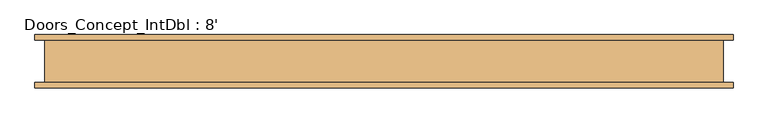
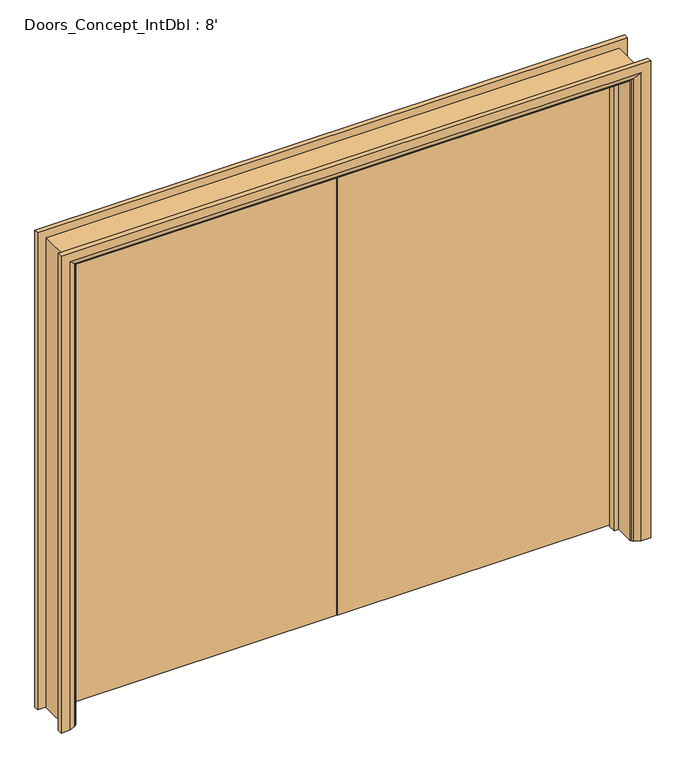
"""IFC4 building model written with IfcOpenShell, lengths in millimetres: door geometry, Doors_Concept_IntDbl : 8'."""

from ifc_helpers import new_model, si_unit, frame, origin, place, context, project, spatial, polyline, circle_curve, ellipse_curve, outline, extrude, faceted_brep, source, transform, mapped, element, save
from ifc_brep_helpers import plane_surface, cylinder_surface, advanced_brep


def doors_concept_intdbl_8_5090a96f(model_context):
    return source(origin(), model_context, "Body", "SolidModel", [
        extrude(outline(polyline([(2110.0, -1219.2), (0.0, -1219.2), (0.0, -1179.2), (2070.0, -1179.2), (2070.0, 1179.2), (0.0, 1179.2), (0.0, 1219.2), (2110.0, 1219.2), (2110.0, -1219.2)])), frame((0.0, -76.2, 0.0), z_axis=(0.0, 1.0, 0.0), x_axis=(0.0, 0.0, 1.0)), (0.0, 0.0, 1.0), 152.4),
        faceted_brep([(-1160.2, 41.2, 0.0), (-1160.2, 9.2, 0.0), (-1179.2, 9.2, 0.0), (-1179.2, 41.2, 0.0), (-1160.2, 41.2, 2051.0), (-1160.2, 9.2, 2051.0), (-1179.2, 9.2, 2070.0), (-1179.2, 41.2, 2070.0), (1160.2, 41.2, 0.0), (1179.2, 41.2, 0.0), (1179.2, 9.2, 0.0), (1160.2, 9.2, 0.0), (1160.2, 41.2, 2051.0), (1179.2, 41.2, 2070.0), (1179.2, 9.2, 2070.0), (1160.2, 9.2, 2051.0)], [[[0, 1, 2, 3]], [[1, 0, 4, 5]], [[2, 1, 5, 6]], [[3, 2, 6, 7]], [[0, 3, 7, 4]], [[8, 9, 10, 11]], [[12, 13, 9, 8]], [[13, 14, 10, 9]], [[14, 15, 11, 10]], [[15, 12, 8, 11]], [[5, 4, 12, 15]], [[6, 5, 15, 14]], [[7, 6, 14, 13]], [[4, 7, 13, 12]]]),
        advanced_brep(
        [(1254.2, 96.2, 0.0), (1254.2, 76.2, 0.0), (1184.2, 76.2, 0.0), (1188.2, 82.2, 0.0), (1214.2, 96.2, 0.0), (1254.2, 96.2, 2145.0), (1254.2, 76.2, 2145.0), (-1254.2, 76.2, 2145.0), (-1254.2, 76.2, 0.0), (-1184.2, 76.2, 0.0), (-1184.2, 76.2, 2075.0), (1184.2, 76.2, 2075.0), (1188.2, 82.2, 2079.0), (1214.2, 96.2, 2105.0), (-1214.2, 96.2, 2105.0), (-1214.2, 96.2, 0.0), (-1254.2, 96.2, 0.0), (-1254.2, 96.2, 2145.0), (-1188.2, 82.2, 0.0), (-1188.2, 82.2, 2079.0)],
        [
            (0, 1),
            (1, 2),
            (2, 3, circle_curve(frame((1192.2, 75.2, 0.0), z_axis=(0.0, 0.0, -1.0), x_axis=(1.0, 0.0, 0.0)), 8.0622577)),
            (3, 4),
            (4, 0),
            (0, 5),
            (5, 6),
            (6, 1),
            (6, 7),
            (7, 8),
            (8, 9),
            (9, 10),
            (10, 11),
            (11, 2),
            (11, 12, ellipse_curve(frame((1192.2, 75.2, 2083.0), z_axis=(0.7071067811865475, 0.0, -0.7071067811865475), x_axis=(-0.7071067811865474, 0.0, -0.7071067811865476)), 11.4017543, 8.0622577)),
            (12, 3),
            (12, 13),
            (13, 4),
            (13, 14),
            (14, 15),
            (15, 16),
            (16, 17),
            (17, 5),
            (7, 17),
            (16, 8),
            (15, 18),
            (18, 9, circle_curve(frame((-1192.2, 75.2, 0.0), z_axis=(0.0, 0.0, -1.0), x_axis=(-1.0, 0.0, 0.0)), 8.0622577)),
            (19, 10, ellipse_curve(frame((-1192.2, 75.2, 2083.0), z_axis=(-0.7071067811865475, 0.0, -0.7071067811865475), x_axis=(-0.7071067811865474, 0.0, 0.7071067811865476)), 11.4017543, 8.0622577)),
            (18, 19),
            (14, 19),
            (19, 12),
        ],
        [
            plane_surface(frame((1184.2, 76.2, 0.0), z_axis=(0.0, 0.0, -1.0), x_axis=(0.0, -1.0, 0.0))),
            plane_surface(frame((1254.2, 96.2, 0.0), z_axis=(1.0, 0.0, 0.0), x_axis=(0.0, 0.0, 1.0))),
            plane_surface(frame((1254.2, 76.2, 0.0), z_axis=(0.0, -1.0, 0.0), x_axis=(0.0, 0.0, 1.0))),
            cylinder_surface(frame((1192.2, 75.2, 0.0), z_axis=(0.0, 0.0, -1.0), x_axis=(1.0, 0.0, 0.0)), 8.0622577),
            plane_surface(frame((1188.2, 82.2, 0.0), z_axis=(-0.4740998230350126, 0.8804710999221779, 0.0), x_axis=(0.0, 0.0, 1.0))),
            plane_surface(frame((1214.2, 96.2, 0.0), z_axis=(0.0, 1.0, 0.0), x_axis=(0.0, 0.0, 1.0))),
            plane_surface(frame((-1254.2, 96.2, 2145.0), z_axis=(-1.0, 0.0, 0.0), x_axis=(0.0, 0.0, -1.0))),
            plane_surface(frame((-1184.2, 76.2, 0.0), z_axis=(0.0, 0.0, -1.0), x_axis=(0.0, -1.0, 0.0))),
            cylinder_surface(frame((-1192.2, 75.2, 2075.0), z_axis=(0.0, 0.0, 1.0), x_axis=(-1.0, 0.0, 0.0)), 8.0622577),
            plane_surface(frame((-1188.2, 82.2, 2079.0), z_axis=(0.4740998230350183, 0.8804710999221749, 0.0), x_axis=(0.0, 0.0, -1.0))),
            plane_surface(frame((1254.2, 96.2, 2145.0), z_axis=(0.0, 0.0, 1.0), x_axis=(-1.0, 0.0, 0.0))),
            cylinder_surface(frame((1184.2, 75.2, 2083.0), z_axis=(1.0, 0.0, 0.0), x_axis=(0.0, 0.0, 1.0)), 8.0622577),
            plane_surface(frame((1188.2, 82.2, 2079.0), z_axis=(0.0, 0.8804710999221763, -0.4740998230350154), x_axis=(-1.0, 0.0, 0.0))),
        ],
        [
            (0, [[1, 2, 3, 4, 5]]),
            (1, [[-1, 6, 7, 8]]),
            (2, [[-2, -8, 9, 10, 11, 12, 13, 14]]),
            (3, [[-3, -14, 15, 16]]),
            (4, [[-4, -16, 17, 18]]),
            (5, [[-5, -18, 19, 20, 21, 22, 23, -6]]),
            (6, [[24, -22, 25, -10]]),
            (7, [[-21, 26, 27, -11, -25]]),
            (8, [[28, -12, -27, 29]]),
            (9, [[30, -29, -26, -20]]),
            (10, [[-7, -23, -24, -9]]),
            (11, [[-15, -13, -28, 31]]),
            (12, [[-17, -31, -30, -19]]),
        ],
    ),
        advanced_brep(
        [(-1254.2, -96.2, 0.0), (-1254.2, -76.2, 0.0), (-1184.2, -76.2, 0.0), (-1188.2, -82.2, 0.0), (-1214.2, -96.2, 0.0), (-1254.2, -96.2, 2145.0), (-1254.2, -76.2, 2145.0), (1254.2, -76.2, 2145.0), (1254.2, -76.2, 0.0), (1184.2, -76.2, 0.0), (1184.2, -76.2, 2075.0), (-1184.2, -76.2, 2075.0), (-1188.2, -82.2, 2079.0), (-1214.2, -96.2, 2105.0), (1214.2, -96.2, 2105.0), (1214.2, -96.2, 0.0), (1254.2, -96.2, 0.0), (1254.2, -96.2, 2145.0), (1188.2, -82.2, 0.0), (1188.2, -82.2, 2079.0)],
        [
            (0, 1),
            (1, 2),
            (2, 3, circle_curve(frame((-1192.2, -75.2, 0.0), z_axis=(0.0, 0.0, -1.0), x_axis=(-1.0, 0.0, 0.0)), 8.0622577)),
            (3, 4),
            (4, 0),
            (0, 5),
            (5, 6),
            (6, 1),
            (6, 7),
            (7, 8),
            (8, 9),
            (9, 10),
            (10, 11),
            (11, 2),
            (11, 12, ellipse_curve(frame((-1192.2, -75.2, 2083.0), z_axis=(-0.7071067811865475, 0.0, -0.7071067811865475), x_axis=(0.7071067811865474, 0.0, -0.7071067811865476)), 11.4017543, 8.0622577)),
            (12, 3),
            (12, 13),
            (13, 4),
            (13, 14),
            (14, 15),
            (15, 16),
            (16, 17),
            (17, 5),
            (7, 17),
            (16, 8),
            (15, 18),
            (18, 9, circle_curve(frame((1192.2, -75.2, 0.0), z_axis=(0.0, 0.0, -1.0), x_axis=(1.0, 0.0, 0.0)), 8.0622577)),
            (19, 10, ellipse_curve(frame((1192.2, -75.2, 2083.0), z_axis=(0.7071067811865475, 0.0, -0.7071067811865475), x_axis=(0.7071067811865474, 0.0, 0.7071067811865476)), 11.4017543, 8.0622577)),
            (18, 19),
            (14, 19),
            (19, 12),
        ],
        [
            plane_surface(frame((-1184.2, -76.2, 0.0), z_axis=(0.0, 0.0, -1.0), x_axis=(0.0, -1.0, 0.0))),
            plane_surface(frame((-1254.2, -96.2, 0.0), z_axis=(-1.0, 0.0, 0.0), x_axis=(0.0, 0.0, 1.0))),
            plane_surface(frame((-1254.2, -76.2, 0.0), z_axis=(0.0, 1.0, 0.0), x_axis=(0.0, 0.0, 1.0))),
            cylinder_surface(frame((-1192.2, -75.2, 0.0), z_axis=(0.0, 0.0, -1.0), x_axis=(-1.0, 0.0, 0.0)), 8.0622577),
            plane_surface(frame((-1188.2, -82.2, 0.0), z_axis=(0.4740998230350183, -0.8804710999221749, 0.0), x_axis=(0.0, 0.0, 1.0))),
            plane_surface(frame((-1214.2, -96.2, 0.0), z_axis=(0.0, -1.0, 0.0), x_axis=(0.0, 0.0, 1.0))),
            plane_surface(frame((1254.2, -96.2, 2145.0), z_axis=(1.0, 0.0, 0.0), x_axis=(0.0, 0.0, -1.0))),
            plane_surface(frame((1184.2, -76.2, 0.0), z_axis=(0.0, 0.0, -1.0), x_axis=(0.0, -1.0, 0.0))),
            cylinder_surface(frame((1192.2, -75.2, 2075.0), z_axis=(0.0, 0.0, 1.0), x_axis=(1.0, 0.0, 0.0)), 8.0622577),
            plane_surface(frame((1188.2, -82.2, 2079.0), z_axis=(-0.4740998230350183, -0.8804710999221749, 0.0), x_axis=(0.0, 0.0, -1.0))),
            plane_surface(frame((-1254.2, -96.2, 2145.0), z_axis=(0.0, 0.0, 1.0), x_axis=(1.0, 0.0, 0.0))),
            cylinder_surface(frame((-1184.2, -75.2, 2083.0), z_axis=(-1.0, 0.0, 0.0), x_axis=(0.0, 0.0, 1.0)), 8.0622577),
            plane_surface(frame((-1188.2, -82.2, 2079.0), z_axis=(0.0, -0.8804710999221749, -0.4740998230350183), x_axis=(1.0, 0.0, 0.0))),
        ],
        [
            (0, [[1, 2, 3, 4, 5]]),
            (1, [[-1, 6, 7, 8]]),
            (2, [[-2, -8, 9, 10, 11, 12, 13, 14]]),
            (3, [[-3, -14, 15, 16]]),
            (4, [[-4, -16, 17, 18]]),
            (5, [[-5, -18, 19, 20, 21, 22, 23, -6]]),
            (6, [[24, -22, 25, -10]]),
            (7, [[-21, 26, 27, -11, -25]]),
            (8, [[28, -12, -27, 29]]),
            (9, [[30, -29, -26, -20]]),
            (10, [[-7, -23, -24, -9]]),
            (11, [[-15, -13, -28, 31]]),
            (12, [[-17, -31, -30, -19]]),
        ],
    ),
        extrude(outline(polyline([(1176.2, 44.2), (1.5, 44.2), (1.5, 76.2), (1176.2, 76.2), (1176.2, 44.2)])), frame((0.0, 0.0, 5.753223), z_axis=(0.0, 0.0, 1.0), x_axis=(1.0, 0.0, 0.0)), (0.0, 0.0, 1.0), 2061.246777),
        extrude(outline(polyline([(-1.5, 44.2), (-1176.2, 44.2), (-1176.2, 76.2), (-1.5, 76.2), (-1.5, 44.2)])), frame((0.0, 0.0, 5.753223), z_axis=(0.0, 0.0, 1.0), x_axis=(1.0, 0.0, 0.0)), (0.0, 0.0, 1.0), 2061.246777),
    ])


if __name__ == "__main__":
    model = new_model("IFC4")
    model_context = context("Model", 3, world=origin())
    ifc_project = project(units=[si_unit("LENGTHUNIT", "METRE", prefix="MILLI")], contexts=[model_context])
    site = spatial("IfcSite", under=ifc_project)
    building = spatial("IfcBuilding", under=site)
    placement = place(None, origin())
    doors_concept_intdbl_8_shape = doors_concept_intdbl_8_5090a96f(model_context)
    element("IfcDoor", 1, ObjectType="Doors_Concept_IntDbl : 8'", at=placement, inside=building, context=model_context, shape_type="MappedRepresentation", body=[
        mapped(doors_concept_intdbl_8_shape, transform((0.0, 0.0, 0.0), x_axis=(1.0, 0.0, 0.0), y_axis=(0.0, 1.0, 0.0), z_axis=(0.0, 0.0, 1.0))),
    ])
    save(model, "model.ifc")

# Revit data of these elements
# Type "Doors_Concept_IntDbl : 8'"
#   Type Mark = "53"
#   Type Comments = "Internal Double"
#   Operation = "DoubleDoorSingleSwing"
#   Construction Type Id = "GSP4R"
#   Keynote = "L10"
#   Description = "Internal Double Door"
#   Analytic Construction = "1/8 in Pilkington single glazing"
#   Visual Light Transmittance = 0.9
#   Thickness = 32 mm
#   Solar Heat Gain Coefficient = 0.78
#   Rough Width = 2438.4 mm
#   Rough Height = 2110 mm
#   Height = 2110 mm
#   Width = 2438.4 mm
#   Heat Transfer Coefficient (U) = 3.6886 W/(m²·K)
#   Define Thermal Properties by = 1
#   Function = 1
#   Material Glass = Glass
#   Material Frame = Glass, Clear Glazing
#   Material Door = Glass
#   Material Architrave = Glass
#   Wall Closure = (empty or 0)
#   Assembly Code = ""
# Element 1 (IfcDoor, "Doors_Concept_IntDbl : 8'")
#   Materials on its faces: "Glass", "Glass, Clear Glazing"
# Materials
#   "Glass": class "Glass", colour RGB 0 128 192, transparency 0.9, Description = "Soda Lime Glass", Cost = 0
#   "Glass, Clear Glazing": class "Glass", colour RGB 0 128 192, transparency 0.75, Description = "Clear glazing", Cost = 0
